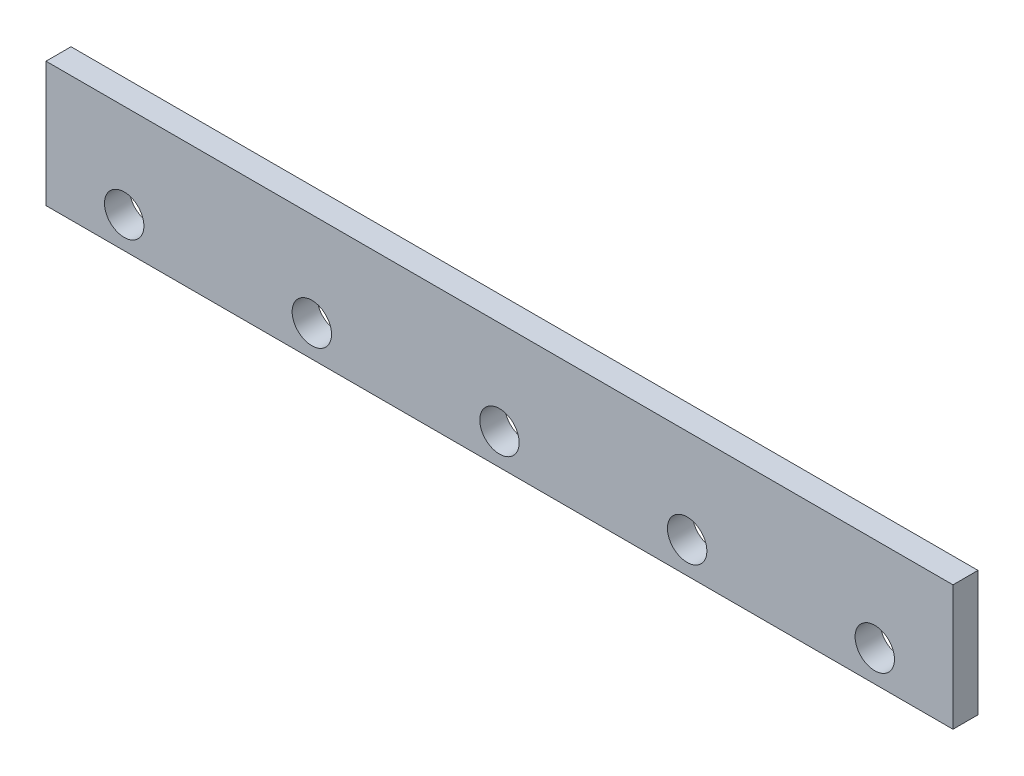
SolidWorks part; units mm, degrees
material "Plain Carbon Steel"
ref_plane "Front Plane" through (0, 0, 0) normal (0, 0, 1) x (1, 0, 0)
ref_plane "Top Plane" through (0, 0, 0) normal (0, 1, 0) x (1, 0, 0)
ref_plane "Right Plane" through (0, 0, 0) normal (1, 0, 0) x (0, 0, -1)
sketch "Bar Profile Sketch" plane through (0, 0, 0) normal (0, 0, 1) x (1, 0, 0)
  line L1 (-290, 40) -> (290, 40)
  line L2 (-290, 40) -> (-290, -40)
  line L3 (-290, -40) -> (290, -40)
  line L4 (290, 40) -> (290, -40)
  line L5 (-290, 40) -> (290, -40) construction
  line L6 (-290, -40) -> (290, 40) construction
  point P0 (0, 0)
  dimension "D1" = 580
  dimension "D2" = 80
extrude "Flat Bar 580x80x16" add sketch "Bar Profile Sketch" along normal blind 16
sketch "Hole Row Sketch" plane through (0, 0, 16) normal (0, 0, 1) x (1, 0, 0)
  line L0 (-290, -40) -> (290, -40) construction
  line L1 (-290, 40) -> (-290, -40) construction
  circle A0 centre (-240, -20) radius 12.6
  circle A1 centre (-120, -20) radius 12.6
  circle A2 centre (0, -20) radius 12.6
  circle A3 centre (120, -20) radius 12.6
  circle A4 centre (240, -20) radius 12.6
  dimension "D3" = 25.2
  dimension "D1" = 20
  dimension "D2" = 50
  dimension "D4" = 120
  dimension "D5" = 120
  dimension "D6" = 120
  dimension "D7" = 120
extrude "Through Holes 5xØ20" cut sketch "Hole Row Sketch" against normal blind 16
